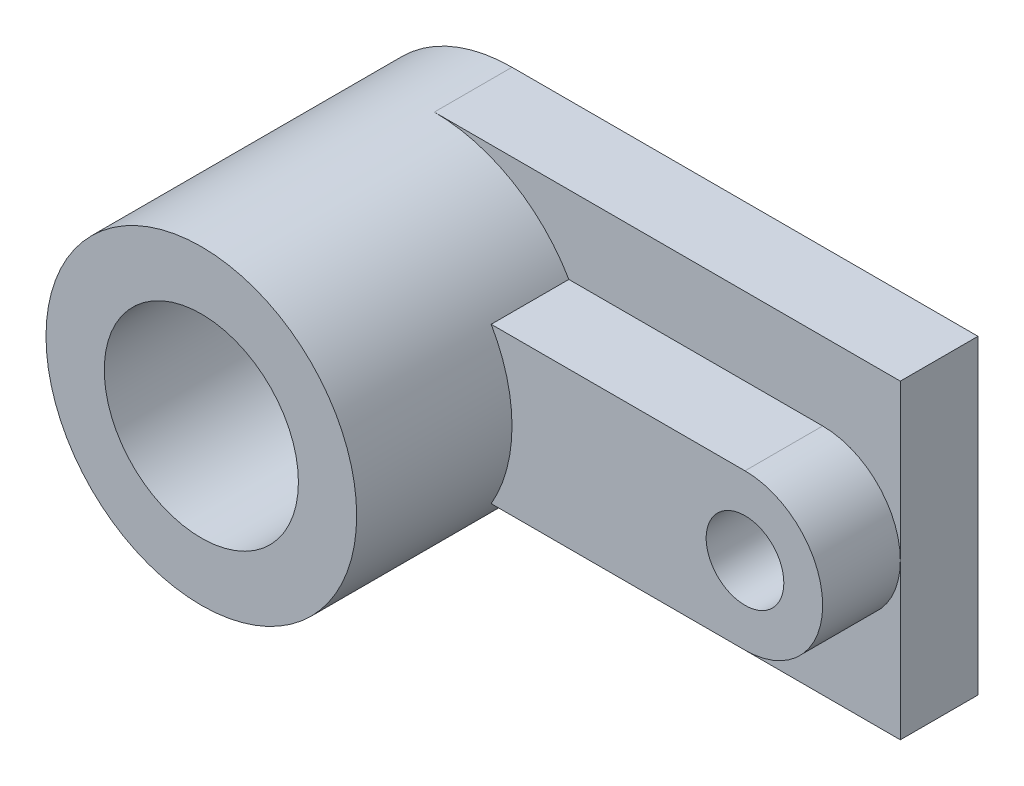
ISO-10303-21;
HEADER;
FILE_DESCRIPTION(('STEP AP214'),'2;1');
FILE_NAME('part.step','',(''),(''),'','','');
FILE_SCHEMA(('AUTOMOTIVE_DESIGN { 1 0 10303 214 1 1 1 1 }'));
ENDSEC;
DATA;
#1=APPLICATION_CONTEXT('core data for automotive mechanical design processes');
#2=APPLICATION_PROTOCOL_DEFINITION('international standard','automotive_design',2000,#1);
#3=PRODUCT_CONTEXT('',#1,'mechanical');
#4=PRODUCT('Part','Part','',(#3));
#5=PRODUCT_RELATED_PRODUCT_CATEGORY('part','',(#4));
#6=PRODUCT_DEFINITION_FORMATION('','',#4);
#7=PRODUCT_DEFINITION_CONTEXT('part definition',#1,'design');
#8=PRODUCT_DEFINITION('design','',#6,#7);
#9=PRODUCT_DEFINITION_SHAPE('','',#8);
#10=(LENGTH_UNIT() NAMED_UNIT(*) SI_UNIT(.MILLI.,.METRE.));
#11=(NAMED_UNIT(*) PLANE_ANGLE_UNIT() SI_UNIT($,.RADIAN.));
#12=(NAMED_UNIT(*) SI_UNIT($,.STERADIAN.) SOLID_ANGLE_UNIT());
#13=UNCERTAINTY_MEASURE_WITH_UNIT(LENGTH_MEASURE(1.E-05),#10,'distance_accuracy_value','');
#14=(GEOMETRIC_REPRESENTATION_CONTEXT(3) GLOBAL_UNCERTAINTY_ASSIGNED_CONTEXT((#13)) GLOBAL_UNIT_ASSIGNED_CONTEXT((#10,
#11,#12)) REPRESENTATION_CONTEXT('',''));
#15=CARTESIAN_POINT('',(0.,0.,0.));
#16=DIRECTION('',(0.,0.,1.));
#17=DIRECTION('',(1.,0.,0.));
#18=AXIS2_PLACEMENT_3D('',#15,#16,#17);
#19=CARTESIAN_POINT('',(0.,-20.,50.));
#20=DIRECTION('',(0.,0.,-1.));
#21=DIRECTION('',(-1.,0.,0.));
#22=AXIS2_PLACEMENT_3D('',#19,#20,#21);
#23=CYLINDRICAL_SURFACE('',#22,20.);
#24=CARTESIAN_POINT('',(0.,-20.,40.));
#25=DIRECTION('',(0.,0.,1.));
#26=DIRECTION('',(1.,0.,0.));
#27=AXIS2_PLACEMENT_3D('',#24,#25,#26);
#28=CIRCLE('',#27,20.);
#29=CARTESIAN_POINT('',(20.,-20.,40.));
#30=VERTEX_POINT('',#29);
#31=EDGE_CURVE('E135',#30,#30,#28,.T.);
#32=ORIENTED_EDGE('',*,*,#31,.F.);
#33=EDGE_LOOP('',(#32));
#34=FACE_BOUND('',#33,.T.);
#35=DIRECTION('',(0.,0.,-1.));
#36=VECTOR('',#35,1.);
#37=CARTESIAN_POINT('',(17.3205080756888,-10.,20.));
#38=LINE('',#37,#36);
#39=CARTESIAN_POINT('',(17.3205080756888,-10.,20.));
#40=VERTEX_POINT('',#39);
#41=CARTESIAN_POINT('',(17.3205080756888,-10.,10.));
#42=VERTEX_POINT('',#41);
#43=EDGE_CURVE('E117',#40,#42,#38,.T.);
#44=ORIENTED_EDGE('',*,*,#43,.T.);
#45=CARTESIAN_POINT('',(0.,-20.,10.));
#46=DIRECTION('',(0.,0.,1.));
#47=DIRECTION('',(1.,0.,0.));
#48=AXIS2_PLACEMENT_3D('',#45,#46,#47);
#49=CIRCLE('',#48,20.);
#50=CARTESIAN_POINT('',(0.,0.,10.));
#51=VERTEX_POINT('',#50);
#52=EDGE_CURVE('E143',#42,#51,#49,.T.);
#53=ORIENTED_EDGE('',*,*,#52,.T.);
#54=DIRECTION('',(0.,0.,-1.));
#55=VECTOR('',#54,1.);
#56=CARTESIAN_POINT('',(0.,0.,10.));
#57=LINE('',#56,#55);
#58=CARTESIAN_POINT('',(0.,0.,0.));
#59=VERTEX_POINT('',#58);
#60=EDGE_CURVE('E157',#51,#59,#57,.T.);
#61=ORIENTED_EDGE('',*,*,#60,.T.);
#62=CARTESIAN_POINT('',(0.,-20.,0.));
#63=DIRECTION('',(0.,0.,-1.));
#64=DIRECTION('',(-1.,0.,0.));
#65=AXIS2_PLACEMENT_3D('',#62,#63,#64);
#66=CIRCLE('',#65,20.);
#67=CARTESIAN_POINT('',(0.,-40.,0.));
#68=VERTEX_POINT('',#67);
#69=EDGE_CURVE('E137',#68,#59,#66,.T.);
#70=ORIENTED_EDGE('',*,*,#69,.F.);
#71=DIRECTION('',(0.,0.,-1.));
#72=VECTOR('',#71,1.);
#73=CARTESIAN_POINT('',(0.,-40.,10.));
#74=LINE('',#73,#72);
#75=CARTESIAN_POINT('',(0.,-40.,10.));
#76=VERTEX_POINT('',#75);
#77=EDGE_CURVE('E166',#76,#68,#74,.T.);
#78=ORIENTED_EDGE('',*,*,#77,.F.);
#79=CARTESIAN_POINT('',(17.3205080756888,-30.,10.));
#80=VERTEX_POINT('',#79);
#81=EDGE_CURVE('E52',#76,#80,#49,.T.);
#82=ORIENTED_EDGE('',*,*,#81,.T.);
#83=DIRECTION('',(0.,0.,-1.));
#84=VECTOR('',#83,1.);
#85=CARTESIAN_POINT('',(17.3205080756888,-30.,20.));
#86=LINE('',#85,#84);
#87=CARTESIAN_POINT('',(17.3205080756888,-30.,20.));
#88=VERTEX_POINT('',#87);
#89=EDGE_CURVE('E63',#88,#80,#86,.T.);
#90=ORIENTED_EDGE('',*,*,#89,.F.);
#91=CARTESIAN_POINT('',(0.,-20.,20.));
#92=DIRECTION('',(0.,0.,-1.));
#93=DIRECTION('',(1.,0.,0.));
#94=AXIS2_PLACEMENT_3D('',#91,#92,#93);
#95=CIRCLE('',#94,20.);
#96=EDGE_CURVE('E58',#40,#88,#95,.T.);
#97=ORIENTED_EDGE('',*,*,#96,.F.);
#98=EDGE_LOOP('',(#44,#53,#61,#70,#78,#82,#90,#97));
#99=FACE_BOUND('',#98,.T.);
#100=ADVANCED_FACE('F44',(#34,#99),#23,.T.);
#101=CARTESIAN_POINT('',(0.,0.,10.));
#102=DIRECTION('',(0.,0.,-1.));
#103=DIRECTION('',(-1.,0.,0.));
#104=AXIS2_PLACEMENT_3D('',#101,#102,#103);
#105=PLANE('',#104);
#106=DIRECTION('',(-1.,0.,0.));
#107=VECTOR('',#106,1.);
#108=CARTESIAN_POINT('',(50.,-10.,10.));
#109=LINE('',#108,#107);
#110=CARTESIAN_POINT('',(50.,-10.,10.));
#111=VERTEX_POINT('',#110);
#112=EDGE_CURVE('E199',#111,#42,#109,.T.);
#113=ORIENTED_EDGE('',*,*,#112,.F.);
#114=CARTESIAN_POINT('',(50.,-20.,10.));
#115=DIRECTION('',(0.,0.,-1.));
#116=DIRECTION('',(-1.,0.,0.));
#117=AXIS2_PLACEMENT_3D('',#114,#115,#116);
#118=CIRCLE('',#117,10.);
#119=CARTESIAN_POINT('',(60.,-20.,10.));
#120=VERTEX_POINT('',#119);
#121=EDGE_CURVE('E11',#120,#111,#118,.F.);
#122=ORIENTED_EDGE('',*,*,#121,.F.);
#123=DIRECTION('',(0.,1.,0.));
#124=VECTOR('',#123,1.);
#125=CARTESIAN_POINT('',(60.,0.,10.));
#126=LINE('',#125,#124);
#127=CARTESIAN_POINT('',(60.,0.,10.));
#128=VERTEX_POINT('',#127);
#129=EDGE_CURVE('E149',#120,#128,#126,.T.);
#130=ORIENTED_EDGE('',*,*,#129,.T.);
#131=DIRECTION('',(-1.,0.,0.));
#132=VECTOR('',#131,1.);
#133=CARTESIAN_POINT('',(0.,0.,10.));
#134=LINE('',#133,#132);
#135=EDGE_CURVE('E155',#128,#51,#134,.T.);
#136=ORIENTED_EDGE('',*,*,#135,.T.);
#137=ORIENTED_EDGE('',*,*,#52,.F.);
#138=EDGE_LOOP('',(#113,#122,#130,#136,#137));
#139=FACE_BOUND('',#138,.T.);
#140=ADVANCED_FACE('F177',(#139),#105,.F.);
#141=CARTESIAN_POINT('',(50.,-20.,10.));
#142=DIRECTION('',(0.,0.,1.));
#143=DIRECTION('',(1.,0.,0.));
#144=AXIS2_PLACEMENT_3D('',#141,#142,#143);
#145=CIRCLE('',#144,10.);
#146=CARTESIAN_POINT('',(50.,-30.,10.));
#147=VERTEX_POINT('',#146);
#148=EDGE_CURVE('E191',#147,#120,#145,.T.);
#149=ORIENTED_EDGE('',*,*,#148,.F.);
#150=DIRECTION('',(1.,0.,0.));
#151=VECTOR('',#150,1.);
#152=CARTESIAN_POINT('',(50.,-30.,10.));
#153=LINE('',#152,#151);
#154=EDGE_CURVE('E126',#80,#147,#153,.T.);
#155=ORIENTED_EDGE('',*,*,#154,.F.);
#156=ORIENTED_EDGE('',*,*,#81,.F.);
#157=DIRECTION('',(1.,0.,0.));
#158=VECTOR('',#157,1.);
#159=CARTESIAN_POINT('',(60.,-40.,10.));
#160=LINE('',#159,#158);
#161=CARTESIAN_POINT('',(60.,-40.,10.));
#162=VERTEX_POINT('',#161);
#163=EDGE_CURVE('E147',#76,#162,#160,.T.);
#164=ORIENTED_EDGE('',*,*,#163,.T.);
#165=EDGE_CURVE('E148',#162,#120,#126,.T.);
#166=ORIENTED_EDGE('',*,*,#165,.T.);
#167=EDGE_LOOP('',(#149,#155,#156,#164,#166));
#168=FACE_BOUND('',#167,.T.);
#169=ADVANCED_FACE('F192',(#168),#105,.F.);
#170=CARTESIAN_POINT('',(60.,-40.,10.));
#171=DIRECTION('',(0.,1.,0.));
#172=DIRECTION('',(0.,0.,1.));
#173=AXIS2_PLACEMENT_3D('',#170,#171,#172);
#174=PLANE('',#173);
#175=DIRECTION('',(1.,0.,0.));
#176=VECTOR('',#175,1.);
#177=CARTESIAN_POINT('',(60.,-40.,0.));
#178=LINE('',#177,#176);
#179=CARTESIAN_POINT('',(60.,-40.,0.));
#180=VERTEX_POINT('',#179);
#181=EDGE_CURVE('E141',#68,#180,#178,.T.);
#182=ORIENTED_EDGE('',*,*,#181,.T.);
#183=DIRECTION('',(0.,0.,-1.));
#184=VECTOR('',#183,1.);
#185=CARTESIAN_POINT('',(60.,-40.,10.));
#186=LINE('',#185,#184);
#187=EDGE_CURVE('E168',#162,#180,#186,.T.);
#188=ORIENTED_EDGE('',*,*,#187,.F.);
#189=ORIENTED_EDGE('',*,*,#163,.F.);
#190=ORIENTED_EDGE('',*,*,#77,.T.);
#191=EDGE_LOOP('',(#182,#188,#189,#190));
#192=FACE_BOUND('',#191,.T.);
#193=ADVANCED_FACE('F50',(#192),#174,.F.);
#194=CARTESIAN_POINT('',(60.,0.,10.));
#195=DIRECTION('',(-1.,0.,0.));
#196=DIRECTION('',(0.,0.,1.));
#197=AXIS2_PLACEMENT_3D('',#194,#195,#196);
#198=PLANE('',#197);
#199=DIRECTION('',(0.,1.,0.));
#200=VECTOR('',#199,1.);
#201=CARTESIAN_POINT('',(60.,0.,0.));
#202=LINE('',#201,#200);
#203=CARTESIAN_POINT('',(60.,0.,0.));
#204=VERTEX_POINT('',#203);
#205=EDGE_CURVE('E160',#180,#204,#202,.T.);
#206=ORIENTED_EDGE('',*,*,#205,.T.);
#207=DIRECTION('',(0.,0.,-1.));
#208=VECTOR('',#207,1.);
#209=CARTESIAN_POINT('',(60.,0.,10.));
#210=LINE('',#209,#208);
#211=EDGE_CURVE('E161',#128,#204,#210,.T.);
#212=ORIENTED_EDGE('',*,*,#211,.F.);
#213=ORIENTED_EDGE('',*,*,#129,.F.);
#214=ORIENTED_EDGE('',*,*,#165,.F.);
#215=ORIENTED_EDGE('',*,*,#187,.T.);
#216=EDGE_LOOP('',(#206,#212,#213,#214,#215));
#217=FACE_BOUND('',#216,.T.);
#218=ADVANCED_FACE('F183',(#217),#198,.F.);
#219=CARTESIAN_POINT('',(0.,0.,10.));
#220=DIRECTION('',(0.,-1.,0.));
#221=DIRECTION('',(0.,0.,-1.));
#222=AXIS2_PLACEMENT_3D('',#219,#220,#221);
#223=PLANE('',#222);
#224=DIRECTION('',(-1.,0.,0.));
#225=VECTOR('',#224,1.);
#226=CARTESIAN_POINT('',(0.,0.,0.));
#227=LINE('',#226,#225);
#228=EDGE_CURVE('E146',#204,#59,#227,.T.);
#229=ORIENTED_EDGE('',*,*,#228,.T.);
#230=ORIENTED_EDGE('',*,*,#60,.F.);
#231=ORIENTED_EDGE('',*,*,#135,.F.);
#232=ORIENTED_EDGE('',*,*,#211,.T.);
#233=EDGE_LOOP('',(#229,#230,#231,#232));
#234=FACE_BOUND('',#233,.T.);
#235=ADVANCED_FACE('F180',(#234),#223,.F.);
#236=CARTESIAN_POINT('',(0.,0.,0.));
#237=DIRECTION('',(0.,0.,-1.));
#238=DIRECTION('',(-1.,0.,0.));
#239=AXIS2_PLACEMENT_3D('',#236,#237,#238);
#240=PLANE('',#239);
#241=ORIENTED_EDGE('',*,*,#181,.F.);
#242=ORIENTED_EDGE('',*,*,#69,.T.);
#243=ORIENTED_EDGE('',*,*,#228,.F.);
#244=ORIENTED_EDGE('',*,*,#205,.F.);
#245=EDGE_LOOP('',(#241,#242,#243,#244));
#246=FACE_BOUND('',#245,.T.);
#247=ADVANCED_FACE('F189',(#246),#240,.T.);
#248=CARTESIAN_POINT('',(0.,-20.,40.));
#249=DIRECTION('',(0.,0.,1.));
#250=DIRECTION('',(1.,0.,0.));
#251=AXIS2_PLACEMENT_3D('',#248,#249,#250);
#252=PLANE('',#251);
#253=CARTESIAN_POINT('',(0.,-20.,40.));
#254=DIRECTION('',(0.,0.,1.));
#255=DIRECTION('',(1.,0.,0.));
#256=AXIS2_PLACEMENT_3D('',#253,#254,#255);
#257=CIRCLE('',#256,12.5);
#258=CARTESIAN_POINT('',(12.5,-20.,40.));
#259=VERTEX_POINT('',#258);
#260=EDGE_CURVE('E214',#259,#259,#257,.T.);
#261=ORIENTED_EDGE('',*,*,#260,.F.);
#262=EDGE_LOOP('',(#261));
#263=FACE_BOUND('',#262,.T.);
#264=ORIENTED_EDGE('',*,*,#31,.T.);
#265=EDGE_LOOP('',(#264));
#266=FACE_BOUND('',#265,.T.);
#267=ADVANCED_FACE('F226',(#263,#266),#252,.T.);
#268=CARTESIAN_POINT('',(50.,-20.,20.));
#269=DIRECTION('',(0.,0.,-1.));
#270=DIRECTION('',(-1.,0.,0.));
#271=AXIS2_PLACEMENT_3D('',#268,#269,#270);
#272=CYLINDRICAL_SURFACE('',#271,10.);
#273=ORIENTED_EDGE('',*,*,#148,.T.);
#274=ORIENTED_EDGE('',*,*,#121,.T.);
#275=DIRECTION('',(0.,0.,-1.));
#276=VECTOR('',#275,1.);
#277=CARTESIAN_POINT('',(50.,-10.,20.));
#278=LINE('',#277,#276);
#279=CARTESIAN_POINT('',(50.,-10.,20.));
#280=VERTEX_POINT('',#279);
#281=EDGE_CURVE('E120',#280,#111,#278,.T.);
#282=ORIENTED_EDGE('',*,*,#281,.F.);
#283=CARTESIAN_POINT('',(50.,-20.,20.));
#284=DIRECTION('',(0.,0.,1.));
#285=DIRECTION('',(1.,0.,0.));
#286=AXIS2_PLACEMENT_3D('',#283,#284,#285);
#287=CIRCLE('',#286,10.);
#288=CARTESIAN_POINT('',(50.,-30.,20.));
#289=VERTEX_POINT('',#288);
#290=EDGE_CURVE('E119',#289,#280,#287,.T.);
#291=ORIENTED_EDGE('',*,*,#290,.F.);
#292=DIRECTION('',(0.,0.,-1.));
#293=VECTOR('',#292,1.);
#294=CARTESIAN_POINT('',(50.,-30.,20.));
#295=LINE('',#294,#293);
#296=EDGE_CURVE('E193',#289,#147,#295,.T.);
#297=ORIENTED_EDGE('',*,*,#296,.T.);
#298=EDGE_LOOP('',(#273,#274,#282,#291,#297));
#299=FACE_BOUND('',#298,.T.);
#300=ADVANCED_FACE('F131',(#299),#272,.T.);
#301=CARTESIAN_POINT('',(50.,-10.,20.));
#302=DIRECTION('',(0.,-1.,0.));
#303=DIRECTION('',(0.,0.,-1.));
#304=AXIS2_PLACEMENT_3D('',#301,#302,#303);
#305=PLANE('',#304);
#306=ORIENTED_EDGE('',*,*,#112,.T.);
#307=ORIENTED_EDGE('',*,*,#43,.F.);
#308=DIRECTION('',(-1.,0.,0.));
#309=VECTOR('',#308,1.);
#310=CARTESIAN_POINT('',(50.,-10.,20.));
#311=LINE('',#310,#309);
#312=EDGE_CURVE('E115',#280,#40,#311,.T.);
#313=ORIENTED_EDGE('',*,*,#312,.F.);
#314=ORIENTED_EDGE('',*,*,#281,.T.);
#315=EDGE_LOOP('',(#306,#307,#313,#314));
#316=FACE_BOUND('',#315,.T.);
#317=ADVANCED_FACE('F114',(#316),#305,.F.);
#318=CARTESIAN_POINT('',(50.,-30.,20.));
#319=DIRECTION('',(0.,1.,0.));
#320=DIRECTION('',(0.,0.,1.));
#321=AXIS2_PLACEMENT_3D('',#318,#319,#320);
#322=PLANE('',#321);
#323=ORIENTED_EDGE('',*,*,#154,.T.);
#324=ORIENTED_EDGE('',*,*,#296,.F.);
#325=DIRECTION('',(1.,0.,0.));
#326=VECTOR('',#325,1.);
#327=CARTESIAN_POINT('',(50.,-30.,20.));
#328=LINE('',#327,#326);
#329=EDGE_CURVE('E123',#88,#289,#328,.T.);
#330=ORIENTED_EDGE('',*,*,#329,.F.);
#331=ORIENTED_EDGE('',*,*,#89,.T.);
#332=EDGE_LOOP('',(#323,#324,#330,#331));
#333=FACE_BOUND('',#332,.T.);
#334=ADVANCED_FACE('F206',(#333),#322,.F.);
#335=CARTESIAN_POINT('',(50.,-20.,20.));
#336=DIRECTION('',(0.,0.,1.));
#337=DIRECTION('',(1.,0.,0.));
#338=AXIS2_PLACEMENT_3D('',#335,#336,#337);
#339=PLANE('',#338);
#340=CARTESIAN_POINT('',(50.,-20.,20.));
#341=DIRECTION('',(0.,0.,1.));
#342=DIRECTION('',(1.,0.,0.));
#343=AXIS2_PLACEMENT_3D('',#340,#341,#342);
#344=CIRCLE('',#343,5.);
#345=CARTESIAN_POINT('',(55.,-20.,20.));
#346=VERTEX_POINT('',#345);
#347=EDGE_CURVE('E202',#346,#346,#344,.T.);
#348=ORIENTED_EDGE('',*,*,#347,.F.);
#349=EDGE_LOOP('',(#348));
#350=FACE_BOUND('',#349,.T.);
#351=ORIENTED_EDGE('',*,*,#290,.T.);
#352=ORIENTED_EDGE('',*,*,#312,.T.);
#353=ORIENTED_EDGE('',*,*,#96,.T.);
#354=ORIENTED_EDGE('',*,*,#329,.T.);
#355=EDGE_LOOP('',(#351,#352,#353,#354));
#356=FACE_BOUND('',#355,.T.);
#357=ADVANCED_FACE('F124',(#350,#356),#339,.T.);
#358=CARTESIAN_POINT('',(50.,-20.,10.));
#359=DIRECTION('',(0.,0.,1.));
#360=DIRECTION('',(1.,0.,0.));
#361=AXIS2_PLACEMENT_3D('',#358,#359,#360);
#362=CYLINDRICAL_SURFACE('',#361,5.);
#363=CARTESIAN_POINT('',(50.,-20.,10.));
#364=DIRECTION('',(0.,0.,1.));
#365=DIRECTION('',(1.,0.,0.));
#366=AXIS2_PLACEMENT_3D('',#363,#364,#365);
#367=CIRCLE('',#366,5.);
#368=CARTESIAN_POINT('',(55.,-20.,10.));
#369=VERTEX_POINT('',#368);
#370=EDGE_CURVE('E196',#369,#369,#367,.T.);
#371=ORIENTED_EDGE('',*,*,#370,.F.);
#372=EDGE_LOOP('',(#371));
#373=FACE_BOUND('',#372,.T.);
#374=ORIENTED_EDGE('',*,*,#347,.T.);
#375=EDGE_LOOP('',(#374));
#376=FACE_BOUND('',#375,.T.);
#377=ADVANCED_FACE('F332',(#373,#376),#362,.F.);
#378=CARTESIAN_POINT('',(50.,-20.,10.));
#379=DIRECTION('',(0.,0.,1.));
#380=DIRECTION('',(1.,0.,0.));
#381=AXIS2_PLACEMENT_3D('',#378,#379,#380);
#382=PLANE('',#381);
#383=ORIENTED_EDGE('',*,*,#370,.T.);
#384=EDGE_LOOP('',(#383));
#385=FACE_BOUND('',#384,.T.);
#386=ADVANCED_FACE('F221',(#385),#382,.T.);
#387=CARTESIAN_POINT('',(0.,-20.,10.));
#388=DIRECTION('',(0.,0.,1.));
#389=DIRECTION('',(1.,0.,0.));
#390=AXIS2_PLACEMENT_3D('',#387,#388,#389);
#391=CYLINDRICAL_SURFACE('',#390,12.5);
#392=CARTESIAN_POINT('',(0.,-20.,10.));
#393=DIRECTION('',(0.,0.,1.));
#394=DIRECTION('',(1.,0.,0.));
#395=AXIS2_PLACEMENT_3D('',#392,#393,#394);
#396=CIRCLE('',#395,12.5);
#397=CARTESIAN_POINT('',(12.5,-20.,10.));
#398=VERTEX_POINT('',#397);
#399=EDGE_CURVE('E212',#398,#398,#396,.T.);
#400=ORIENTED_EDGE('',*,*,#399,.F.);
#401=EDGE_LOOP('',(#400));
#402=FACE_BOUND('',#401,.T.);
#403=ORIENTED_EDGE('',*,*,#260,.T.);
#404=EDGE_LOOP('',(#403));
#405=FACE_BOUND('',#404,.T.);
#406=ADVANCED_FACE('F222',(#402,#405),#391,.F.);
#407=CARTESIAN_POINT('',(0.,-20.,10.));
#408=DIRECTION('',(0.,0.,1.));
#409=DIRECTION('',(1.,0.,0.));
#410=AXIS2_PLACEMENT_3D('',#407,#408,#409);
#411=PLANE('',#410);
#412=ORIENTED_EDGE('',*,*,#399,.T.);
#413=EDGE_LOOP('',(#412));
#414=FACE_BOUND('',#413,.T.);
#415=ADVANCED_FACE('F218',(#414),#411,.T.);
#416=CLOSED_SHELL('',(#100,#140,#169,#193,#218,#235,#247,#267,#300,#317,#334,#357,#377,#386,
#406,#415));
#417=MANIFOLD_SOLID_BREP('B2',#416);
#418=ADVANCED_BREP_SHAPE_REPRESENTATION('',(#18,#417),#14);
#419=SHAPE_DEFINITION_REPRESENTATION(#9,#418);
ENDSEC;
END-ISO-10303-21;
